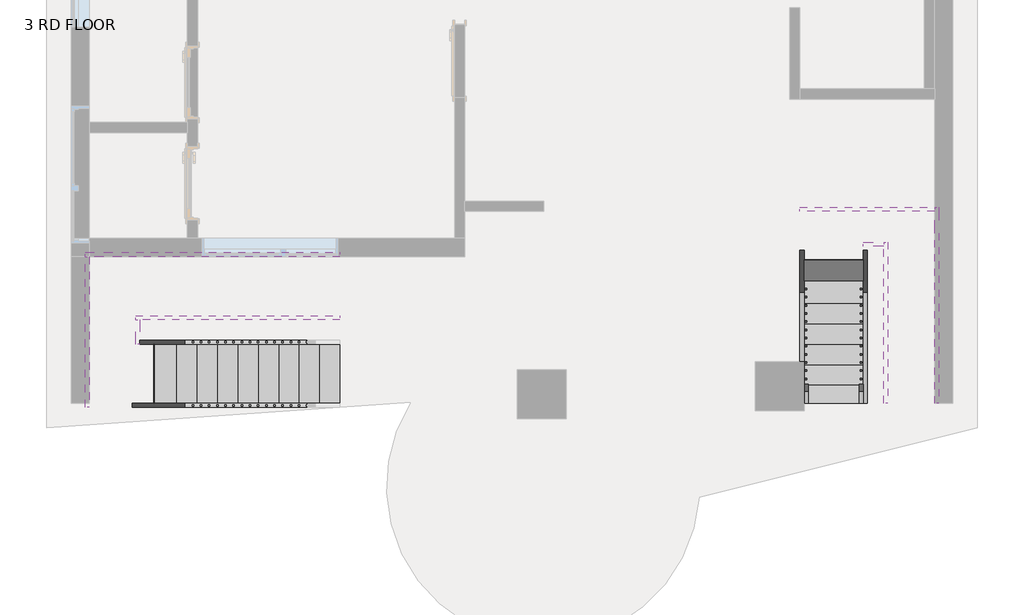
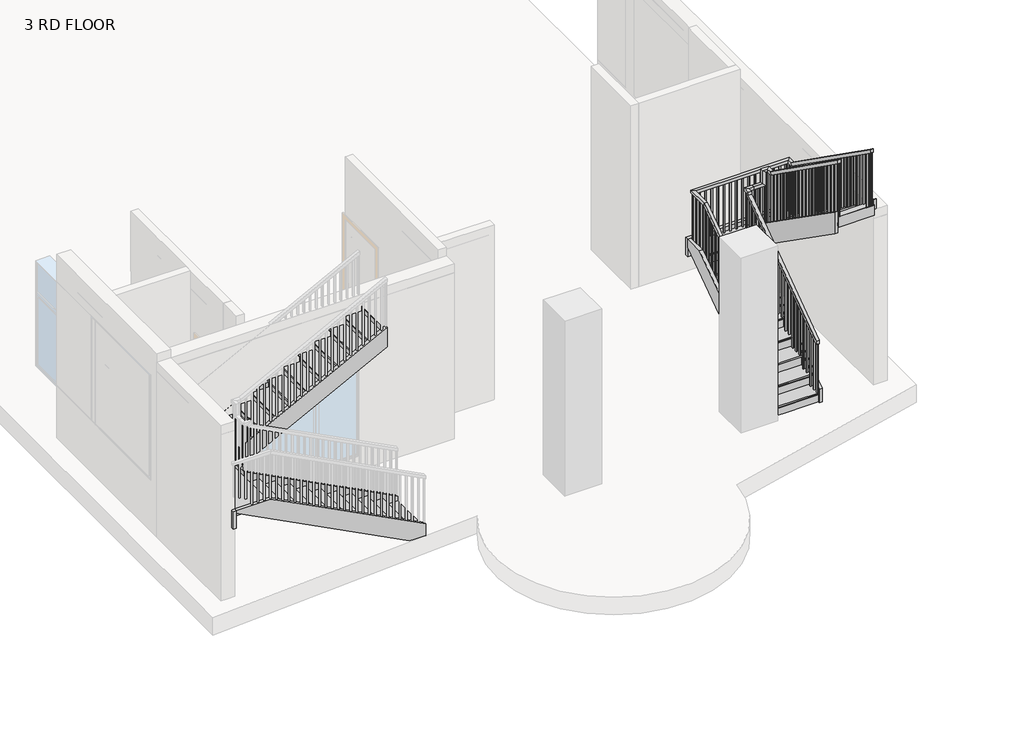
# One storey, part 5 of 5: 12 members, 2 railings, 2 stair flights.
"""IFC4 building model written with IfcOpenShell, lengths in millimetres."""

from ifc_helpers import new_model, si_unit, frame, origin, place, context, project, spatial, polyline, outline, extrude, faceted_brep, transform, mapped, element, save
from components import stair_flight_862ef343, stair_flight_4914edaa

model = new_model("IFC4")

# Units and contexts
model_context = context("Model", 3, world=origin())
ifc_project = project(units=[si_unit("LENGTHUNIT", "METRE", prefix="MILLI")], contexts=[model_context])

# Site, building, storey
site = spatial("IfcSite", under=ifc_project)
building = spatial("IfcBuilding", under=site)
storey = spatial("IfcBuildingStorey", under=building, Name="3 RD FLOOR", Elevation=9601.2)

# Members
placement = place(None, origin())
element("IfcMember", 1, ObjectType="Stringer - 2\" Width", at=placement, inside=storey, context=model_context, shape_type="SweptSolid", body=[
    extrude(outline(polyline([(9601.2, -3117.2664982), (9805.7197081, -3117.2664982), (11125.2, -5663.6319738), (11125.2, -6232.5131972), (11076.6929835, -6232.5131972), (9601.2, -3385.0705974), (9601.2, -3117.2664982)])), frame((0.0, -7701.7822004, 0.0), z_axis=(0.0, 1.0, 0.0), x_axis=(0.0, 0.0, 1.0)), (0.0, 0.0, 1.0), 50.8),
])
element("IfcMember", 2, ObjectType="Stringer - 2\" Width", at=placement, inside=storey, context=model_context, shape_type="SweptSolid", body=[
    extrude(outline(polyline([(-6232.5131972, -7701.7822004), (-6283.3131972, -7701.7822004), (-6283.3131972, -5824.7082131), (-6232.5131972, -5824.7082131), (-6232.5131972, -7701.7822004)])), frame((0.0, 0.0, 10820.4), z_axis=(0.0, 0.0, 1.0), x_axis=(1.0, 0.0, 0.0)), (0.0, 0.0, 1.0), 304.8),
])
element("IfcMember", 3, ObjectType="Stringer - 2\" Width", at=placement, inside=storey, context=model_context, shape_type="SweptSolid", body=[
    extrude(outline(polyline([(10929.1136913, -6283.3131972), (10820.4, -6283.3131972), (10820.4, -5830.6202937), (12226.4106031, -3117.2664982), (12569.7015263, -3117.2664982), (10929.1136913, -6283.3131972)])), frame((0.0, -5824.7082131, 0.0), z_axis=(0.0, 1.0, 0.0), x_axis=(0.0, 0.0, 1.0)), (0.0, 0.0, 1.0), 50.8),
])
element("IfcMember", 4, ObjectType="Stringer - 2\" Width", at=placement, inside=storey, context=model_context, shape_type="SweptSolid", body=[
    extrude(outline(polyline([(9601.2, -3117.2664982), (9805.7197081, -3117.2664982), (11095.5778899, -5606.4664982), (10752.2869668, -5606.4664982), (9601.2, -3385.0705974), (9601.2, -3117.2664982)])), frame((0.0, -6914.3822004, 0.0), z_axis=(0.0, 1.0, 0.0), x_axis=(0.0, 0.0, 1.0)), (0.0, 0.0, 1.0), 50.8),
])
element("IfcMember", 5, ObjectType="Stringer - 2\" Width", at=placement, inside=storey, context=model_context, shape_type="SweptSolid", body=[
    extrude(outline(polyline([(-5606.4664982, -6914.3822004), (-5657.2664982, -6914.3822004), (-5657.2664982, -6609.5822004), (-5606.4664982, -6609.5822004), (-5606.4664982, -6914.3822004)])), frame((0.0, 0.0, 10820.4), z_axis=(0.0, 0.0, 1.0), x_axis=(1.0, 0.0, 0.0)), (0.0, 0.0, 1.0), 304.8),
])
element("IfcMember", 6, ObjectType="Stringer - 2\" Width", at=placement, inside=storey, context=model_context, shape_type="SweptSolid", body=[
    extrude(outline(polyline([(11253.5197081, -5657.2664982), (10910.2287849, -5657.2664982), (12226.4106031, -3117.2664982), (12569.7015263, -3117.2664982), (11253.5197081, -5657.2664982)])), frame((0.0, -6609.5822004, 0.0), z_axis=(0.0, 1.0, 0.0), x_axis=(0.0, 0.0, 1.0)), (0.0, 0.0, 1.0), 50.8),
])
element("IfcMember", 7, ObjectType="Stringer - 2\" Width", at=placement, inside=storey, context=model_context, shape_type="SweptSolid", body=[
    extrude(outline(polyline([(-7650.9822004, 9601.2), (-7650.9822004, 9840.499187), (-5597.981039, 11277.6), (-5263.3822004, 11277.6), (-5263.3822004, 11139.7633718), (-7461.3298744, 9601.2), (-7650.9822004, 9601.2)])), frame((2606.6891134, 0.0, 0.0), z_axis=(1.0, 0.0, 0.0), x_axis=(0.0, 1.0, 0.0)), (0.0, 0.0, 1.0), 50.8),
])
element("IfcMember", 8, ObjectType="Stringer - 2\" Width", at=placement, inside=storey, context=model_context, shape_type="SweptSolid", body=[
    extrude(outline(polyline([(2606.6891134, -5263.3822004), (2606.6891134, -5212.5822004), (4281.7311655, -5212.5822004), (4281.7311655, -5263.3822004), (2606.6891134, -5263.3822004)])), frame((0.0, 0.0, 10972.8), z_axis=(0.0, 0.0, 1.0), x_axis=(1.0, 0.0, 0.0)), (0.0, 0.0, 1.0), 304.8),
])
element("IfcMember", 9, ObjectType="Stringer - 2\" Width", at=placement, inside=storey, context=model_context, shape_type="SweptSolid", body=[
    extrude(outline(polyline([(-5212.5822004, 11120.659187), (-5212.5822004, 10972.8), (-5532.8630978, 10972.8), (-7650.9822004, 12455.4833718), (-7650.9822004, 12827.539187), (-5212.5822004, 11120.659187)])), frame((4281.7311655, 0.0, 0.0), z_axis=(1.0, 0.0, 0.0), x_axis=(0.0, 1.0, 0.0)), (0.0, 0.0, 1.0), 50.8),
])
element("IfcMember", 10, ObjectType="Stringer - 2\" Width", at=placement, inside=storey, context=model_context, shape_type="SweptSolid", body=[
    extrude(outline(polyline([(-7650.9822004, 9601.2), (-7650.9822004, 9840.499187), (-5695.1822004, 11209.559187), (-5695.1822004, 10837.5033718), (-7461.3298744, 9601.2), (-7650.9822004, 9601.2)])), frame((3394.0891134, 0.0, 0.0), z_axis=(1.0, 0.0, 0.0), x_axis=(0.0, 1.0, 0.0)), (0.0, 0.0, 1.0), 50.8),
])
element("IfcMember", 11, ObjectType="Stringer - 2\" Width", at=placement, inside=storey, context=model_context, shape_type="SweptSolid", body=[
    extrude(outline(polyline([(3394.0891134, -5695.1822004), (3394.0891134, -5644.3822004), (3648.0891134, -5644.3822004), (3648.0891134, -5695.1822004), (3394.0891134, -5695.1822004)])), frame((0.0, 0.0, 10972.8), z_axis=(0.0, 0.0, 1.0), x_axis=(1.0, 0.0, 0.0)), (0.0, 0.0, 1.0), 304.8),
])
element("IfcMember", 12, ObjectType="Stringer - 2\" Width", at=placement, inside=storey, context=model_context, shape_type="SweptSolid", body=[
    extrude(outline(polyline([(-5644.3822004, 11422.919187), (-5644.3822004, 11050.8633718), (-7650.9822004, 12455.4833718), (-7650.9822004, 12827.539187), (-5644.3822004, 11422.919187)])), frame((3648.0891134, 0.0, 0.0), z_axis=(1.0, 0.0, 0.0), x_axis=(0.0, 1.0, 0.0)), (0.0, 0.0, 1.0), 50.8),
])

# Railings
element("IfcRailing", 13, ObjectType="Handrail - Rectangular", at=placement, inside=storey, context=model_context, shape_type="SolidModel", body=[
    faceted_brep([(3343.2891134, -7650.9822004, 10693.4), (3343.2891134, -7650.9822004, 10631.1314749), (3394.0891134, -7650.9822004, 10631.1314749), (3394.0891134, -7650.9822004, 10693.4), (3343.2891134, -5720.5822004, 12061.7848101), (3343.2891134, -5669.7822004, 12035.5264116), (3394.0891134, -5669.7822004, 12035.5264116), (3394.0891134, -5720.5822004, 12061.7848101), (3343.2891134, -5720.5822004, 12115.8), (3343.2891134, -5669.7822004, 12065.0), (3394.0891134, -5669.7822004, 12065.0), (3394.0891134, -5720.5822004, 12115.8), (3343.2891134, -5593.5822004, 12115.8), (3343.2891134, -5593.5822004, 12065.0), (3394.0891134, -5644.3822004, 12065.0), (3394.0891134, -5644.3822004, 12115.8), (3470.2891134, -5593.5822004, 12115.8), (3470.2891134, -5593.5822004, 12065.0), (3470.2891134, -5644.3822004, 12065.0), (3470.2891134, -5644.3822004, 12115.8), (3622.6891134, -5593.5822004, 12115.8), (3673.4891134, -5593.5822004, 12065.0), (3673.4891134, -5644.3822004, 12065.0), (3622.6891134, -5644.3822004, 12115.8), (3622.6891134, -5593.5822004, 12347.6151899), (3673.4891134, -5593.5822004, 12296.8151899), (3673.4891134, -5644.3822004, 12296.8151899), (3622.6891134, -5644.3822004, 12347.6151899), (3749.6891134, -5593.5822004, 12347.6151899), (3749.6891134, -5593.5822004, 12296.8151899), (3698.8891134, -5644.3822004, 12296.8151899), (3698.8891134, -5644.3822004, 12347.6151899), (3749.6891134, -5720.5822004, 12347.6151899), (3749.6891134, -5736.7610126, 12296.8151899), (3698.8891134, -5736.7610126, 12296.8151899), (3698.8891134, -5720.5822004, 12347.6151899), (3749.6891134, -7650.9822004, 13716.0), (3698.8891134, -7650.9822004, 13716.0), (3698.8891134, -7650.9822004, 13653.7314749), (3749.6891134, -7650.9822004, 13653.7314749)], [[[0, 1, 2, 3]], [[1, 0, 4, 5]], [[2, 1, 5, 6]], [[3, 2, 6, 7]], [[0, 3, 7, 4]], [[5, 4, 8, 9]], [[6, 5, 9, 10]], [[7, 6, 10, 11]], [[4, 7, 11, 8]], [[9, 8, 12, 13]], [[10, 9, 13, 14]], [[11, 10, 14, 15]], [[8, 11, 15, 12]], [[13, 12, 16, 17]], [[14, 13, 17, 18]], [[15, 14, 18, 19]], [[12, 15, 19, 16]], [[17, 16, 20, 21]], [[18, 17, 21, 22]], [[19, 18, 22, 23]], [[16, 19, 23, 20]], [[21, 20, 24, 25]], [[22, 21, 25, 26]], [[23, 22, 26, 27]], [[20, 23, 27, 24]], [[25, 24, 28, 29]], [[26, 25, 29, 30]], [[27, 26, 30, 31]], [[24, 27, 31, 28]], [[29, 28, 32, 33]], [[30, 29, 33, 34]], [[31, 30, 34, 35]], [[28, 31, 35, 32]], [[36, 37, 38, 39]], [[33, 32, 36, 39]], [[34, 33, 39, 38]], [[35, 34, 38, 37]], [[32, 35, 37, 36]]]),
    extrude(outline(polyline([(-7558.9072004, 13588.4631205), (-7539.8572004, 13574.959323), (-7539.8572004, 12623.8), (-7558.9072004, 12623.8), (-7558.9072004, 13588.4631205)])), frame((3714.7641134, 0.0, 0.0), z_axis=(1.0, 0.0, 0.0), x_axis=(0.0, 1.0, 0.0)), (0.0, 0.0, 1.0), 19.05),
    extrude(outline(polyline([(-7457.3072004, 13516.4428673), (-7438.2572004, 13502.9390699), (-7438.2572004, 12623.8), (-7457.3072004, 12623.8), (-7457.3072004, 13516.4428673)])), frame((3714.7641134, 0.0, 0.0), z_axis=(1.0, 0.0, 0.0), x_axis=(0.0, 1.0, 0.0)), (0.0, 0.0, 1.0), 19.05),
    extrude(outline(polyline([(-7355.7072004, 13444.4226142), (-7336.6572004, 13430.9188167), (-7336.6572004, 12446.0), (-7355.7072004, 12446.0), (-7355.7072004, 13444.4226142)])), frame((3714.7641134, 0.0, 0.0), z_axis=(1.0, 0.0, 0.0), x_axis=(0.0, 1.0, 0.0)), (0.0, 0.0, 1.0), 19.05),
    extrude(outline(polyline([(-7254.1072004, 13372.402361), (-7235.0572004, 13358.8985635), (-7235.0572004, 12446.0), (-7254.1072004, 12446.0), (-7254.1072004, 13372.402361)])), frame((3714.7641134, 0.0, 0.0), z_axis=(1.0, 0.0, 0.0), x_axis=(0.0, 1.0, 0.0)), (0.0, 0.0, 1.0), 19.05),
    extrude(outline(polyline([(-7152.5072004, 13300.3821078), (-7133.4572004, 13286.8783104), (-7133.4572004, 12268.2), (-7152.5072004, 12268.2), (-7152.5072004, 13300.3821078)])), frame((3714.7641134, 0.0, 0.0), z_axis=(1.0, 0.0, 0.0), x_axis=(0.0, 1.0, 0.0)), (0.0, 0.0, 1.0), 19.05),
    extrude(outline(polyline([(-7050.9072004, 13228.3618547), (-7031.8572004, 13214.8580572), (-7031.8572004, 12268.2), (-7050.9072004, 12268.2), (-7050.9072004, 13228.3618547)])), frame((3714.7641134, 0.0, 0.0), z_axis=(1.0, 0.0, 0.0), x_axis=(0.0, 1.0, 0.0)), (0.0, 0.0, 1.0), 19.05),
    extrude(outline(polyline([(-6949.3072004, 13156.3416015), (-6930.2572004, 13142.837804), (-6930.2572004, 12268.2), (-6949.3072004, 12268.2), (-6949.3072004, 13156.3416015)])), frame((3714.7641134, 0.0, 0.0), z_axis=(1.0, 0.0, 0.0), x_axis=(0.0, 1.0, 0.0)), (0.0, 0.0, 1.0), 19.05),
    extrude(outline(polyline([(-6847.7072004, 13084.3213483), (-6828.6572004, 13070.8175509), (-6828.6572004, 12090.4), (-6847.7072004, 12090.4), (-6847.7072004, 13084.3213483)])), frame((3714.7641134, 0.0, 0.0), z_axis=(1.0, 0.0, 0.0), x_axis=(0.0, 1.0, 0.0)), (0.0, 0.0, 1.0), 19.05),
    extrude(outline(polyline([(-6746.1072004, 13012.3010952), (-6727.0572004, 12998.7972977), (-6727.0572004, 12090.4), (-6746.1072004, 12090.4), (-6746.1072004, 13012.3010952)])), frame((3714.7641134, 0.0, 0.0), z_axis=(1.0, 0.0, 0.0), x_axis=(0.0, 1.0, 0.0)), (0.0, 0.0, 1.0), 19.05),
    extrude(outline(polyline([(-6644.5072004, 12940.280842), (-6625.4572004, 12926.7770445), (-6625.4572004, 11912.6), (-6644.5072004, 11912.6), (-6644.5072004, 12940.280842)])), frame((3714.7641134, 0.0, 0.0), z_axis=(1.0, 0.0, 0.0), x_axis=(0.0, 1.0, 0.0)), (0.0, 0.0, 1.0), 19.05),
    extrude(outline(polyline([(-6542.9072004, 12868.2605888), (-6523.8572004, 12854.7567914), (-6523.8572004, 11912.6), (-6542.9072004, 11912.6), (-6542.9072004, 12868.2605888)])), frame((3714.7641134, 0.0, 0.0), z_axis=(1.0, 0.0, 0.0), x_axis=(0.0, 1.0, 0.0)), (0.0, 0.0, 1.0), 19.05),
    extrude(outline(polyline([(-6441.3072004, 12796.2403357), (-6422.2572004, 12782.7365382), (-6422.2572004, 11912.6), (-6441.3072004, 11912.6), (-6441.3072004, 12796.2403357)])), frame((3714.7641134, 0.0, 0.0), z_axis=(1.0, 0.0, 0.0), x_axis=(0.0, 1.0, 0.0)), (0.0, 0.0, 1.0), 19.05),
    extrude(outline(polyline([(-6339.7072004, 12724.2200825), (-6320.6572004, 12710.716285), (-6320.6572004, 11734.8), (-6339.7072004, 11734.8), (-6339.7072004, 12724.2200825)])), frame((3714.7641134, 0.0, 0.0), z_axis=(1.0, 0.0, 0.0), x_axis=(0.0, 1.0, 0.0)), (0.0, 0.0, 1.0), 19.05),
    extrude(outline(polyline([(-6238.1072004, 12652.1998293), (-6219.0572004, 12638.6960319), (-6219.0572004, 11734.8), (-6238.1072004, 11734.8), (-6238.1072004, 12652.1998293)])), frame((3714.7641134, 0.0, 0.0), z_axis=(1.0, 0.0, 0.0), x_axis=(0.0, 1.0, 0.0)), (0.0, 0.0, 1.0), 19.05),
    extrude(outline(polyline([(-6136.5072004, 12580.1795762), (-6117.4572004, 12566.6757787), (-6117.4572004, 11557.0), (-6136.5072004, 11557.0), (-6136.5072004, 12580.1795762)])), frame((3714.7641134, 0.0, 0.0), z_axis=(1.0, 0.0, 0.0), x_axis=(0.0, 1.0, 0.0)), (0.0, 0.0, 1.0), 19.05),
    extrude(outline(polyline([(-6034.9072004, 12508.159323), (-6015.8572004, 12494.6555255), (-6015.8572004, 11557.0), (-6034.9072004, 11557.0), (-6034.9072004, 12508.159323)])), frame((3714.7641134, 0.0, 0.0), z_axis=(1.0, 0.0, 0.0), x_axis=(0.0, 1.0, 0.0)), (0.0, 0.0, 1.0), 19.05),
    extrude(outline(polyline([(-5933.3072004, 12436.1390699), (-5914.2572004, 12422.6352724), (-5914.2572004, 11557.0), (-5933.3072004, 11557.0), (-5933.3072004, 12436.1390699)])), frame((3714.7641134, 0.0, 0.0), z_axis=(1.0, 0.0, 0.0), x_axis=(0.0, 1.0, 0.0)), (0.0, 0.0, 1.0), 19.05),
    extrude(outline(polyline([(-5831.7072004, 12364.1188167), (-5812.6572004, 12350.6150192), (-5812.6572004, 11379.2), (-5831.7072004, 11379.2), (-5831.7072004, 12364.1188167)])), frame((3714.7641134, 0.0, 0.0), z_axis=(1.0, 0.0, 0.0), x_axis=(0.0, 1.0, 0.0)), (0.0, 0.0, 1.0), 19.05),
    extrude(outline(polyline([(-5730.1072004, 12292.0985635), (-5711.0572004, 12278.5947661), (-5711.0572004, 11379.2), (-5730.1072004, 11379.2), (-5730.1072004, 12292.0985635)])), frame((3714.7641134, 0.0, 0.0), z_axis=(1.0, 0.0, 0.0), x_axis=(0.0, 1.0, 0.0)), (0.0, 0.0, 1.0), 19.05),
    extrude(outline(polyline([(3663.9641134, -5628.5072004), (3663.9641134, -5609.4572004), (3683.0141134, -5609.4572004), (3683.0141134, -5628.5072004), (3663.9641134, -5628.5072004)])), frame((0.0, 0.0, 11201.4), z_axis=(0.0, 0.0, 1.0), x_axis=(1.0, 0.0, 0.0)), (0.0, 0.0, 1.0), 1095.4151899),
    extrude(outline(polyline([(3562.3641134, -5628.5072004), (3562.3641134, -5609.4572004), (3581.4141134, -5609.4572004), (3581.4141134, -5628.5072004), (3562.3641134, -5628.5072004)])), frame((0.0, 0.0, 11201.4), z_axis=(0.0, 0.0, 1.0), x_axis=(1.0, 0.0, 0.0)), (0.0, 0.0, 1.0), 863.6),
    extrude(outline(polyline([(3460.7641134, -5628.5072004), (3460.7641134, -5609.4572004), (3479.8141134, -5609.4572004), (3479.8141134, -5628.5072004), (3460.7641134, -5628.5072004)])), frame((0.0, 0.0, 11201.4), z_axis=(0.0, 0.0, 1.0), x_axis=(1.0, 0.0, 0.0)), (0.0, 0.0, 1.0), 863.6),
    extrude(outline(polyline([(-5730.1072004, 11992.7643863), (-5711.0572004, 12006.2681838), (-5711.0572004, 11023.6), (-5730.1072004, 11023.6), (-5730.1072004, 11992.7643863)])), frame((3359.1641134, 0.0, 0.0), z_axis=(1.0, 0.0, 0.0), x_axis=(0.0, 1.0, 0.0)), (0.0, 0.0, 1.0), 19.05),
    extrude(outline(polyline([(-5831.7072004, 11920.7441331), (-5812.6572004, 11934.2479306), (-5812.6572004, 11023.6), (-5831.7072004, 11023.6), (-5831.7072004, 11920.7441331)])), frame((3359.1641134, 0.0, 0.0), z_axis=(1.0, 0.0, 0.0), x_axis=(0.0, 1.0, 0.0)), (0.0, 0.0, 1.0), 19.05),
    extrude(outline(polyline([(-5933.3072004, 11848.72388), (-5914.2572004, 11862.2276774), (-5914.2572004, 10845.8), (-5933.3072004, 10845.8), (-5933.3072004, 11848.72388)])), frame((3359.1641134, 0.0, 0.0), z_axis=(1.0, 0.0, 0.0), x_axis=(0.0, 1.0, 0.0)), (0.0, 0.0, 1.0), 19.05),
    extrude(outline(polyline([(-6034.9072004, 11776.7036268), (-6015.8572004, 11790.2074243), (-6015.8572004, 10845.8), (-6034.9072004, 10845.8), (-6034.9072004, 11776.7036268)])), frame((3359.1641134, 0.0, 0.0), z_axis=(1.0, 0.0, 0.0), x_axis=(0.0, 1.0, 0.0)), (0.0, 0.0, 1.0), 19.05),
    extrude(outline(polyline([(-6136.5072004, 11704.6833736), (-6117.4572004, 11718.1871711), (-6117.4572004, 10845.8), (-6136.5072004, 10845.8), (-6136.5072004, 11704.6833736)])), frame((3359.1641134, 0.0, 0.0), z_axis=(1.0, 0.0, 0.0), x_axis=(0.0, 1.0, 0.0)), (0.0, 0.0, 1.0), 19.05),
    extrude(outline(polyline([(-6238.1072004, 11632.6631205), (-6219.0572004, 11646.166918), (-6219.0572004, 10668.0), (-6238.1072004, 10668.0), (-6238.1072004, 11632.6631205)])), frame((3359.1641134, 0.0, 0.0), z_axis=(1.0, 0.0, 0.0), x_axis=(0.0, 1.0, 0.0)), (0.0, 0.0, 1.0), 19.05),
    extrude(outline(polyline([(-6339.7072004, 11560.6428673), (-6320.6572004, 11574.1466648), (-6320.6572004, 10668.0), (-6339.7072004, 10668.0), (-6339.7072004, 11560.6428673)])), frame((3359.1641134, 0.0, 0.0), z_axis=(1.0, 0.0, 0.0), x_axis=(0.0, 1.0, 0.0)), (0.0, 0.0, 1.0), 19.05),
    extrude(outline(polyline([(-6441.3072004, 11488.6226142), (-6422.2572004, 11502.1264116), (-6422.2572004, 10490.2), (-6441.3072004, 10490.2), (-6441.3072004, 11488.6226142)])), frame((3359.1641134, 0.0, 0.0), z_axis=(1.0, 0.0, 0.0), x_axis=(0.0, 1.0, 0.0)), (0.0, 0.0, 1.0), 19.05),
    extrude(outline(polyline([(-6542.9072004, 11416.602361), (-6523.8572004, 11430.1061585), (-6523.8572004, 10490.2), (-6542.9072004, 10490.2), (-6542.9072004, 11416.602361)])), frame((3359.1641134, 0.0, 0.0), z_axis=(1.0, 0.0, 0.0), x_axis=(0.0, 1.0, 0.0)), (0.0, 0.0, 1.0), 19.05),
    extrude(outline(polyline([(-6644.5072004, 11344.5821078), (-6625.4572004, 11358.0859053), (-6625.4572004, 10490.2), (-6644.5072004, 10490.2), (-6644.5072004, 11344.5821078)])), frame((3359.1641134, 0.0, 0.0), z_axis=(1.0, 0.0, 0.0), x_axis=(0.0, 1.0, 0.0)), (0.0, 0.0, 1.0), 19.05),
    extrude(outline(polyline([(-6746.1072004, 11272.5618547), (-6727.0572004, 11286.0656521), (-6727.0572004, 10312.4), (-6746.1072004, 10312.4), (-6746.1072004, 11272.5618547)])), frame((3359.1641134, 0.0, 0.0), z_axis=(1.0, 0.0, 0.0), x_axis=(0.0, 1.0, 0.0)), (0.0, 0.0, 1.0), 19.05),
    extrude(outline(polyline([(-6847.7072004, 11200.5416015), (-6828.6572004, 11214.045399), (-6828.6572004, 10312.4), (-6847.7072004, 10312.4), (-6847.7072004, 11200.5416015)])), frame((3359.1641134, 0.0, 0.0), z_axis=(1.0, 0.0, 0.0), x_axis=(0.0, 1.0, 0.0)), (0.0, 0.0, 1.0), 19.05),
    extrude(outline(polyline([(-6949.3072004, 11128.5213483), (-6930.2572004, 11142.0251458), (-6930.2572004, 10134.6), (-6949.3072004, 10134.6), (-6949.3072004, 11128.5213483)])), frame((3359.1641134, 0.0, 0.0), z_axis=(1.0, 0.0, 0.0), x_axis=(0.0, 1.0, 0.0)), (0.0, 0.0, 1.0), 19.05),
    extrude(outline(polyline([(-7050.9072004, 11056.5010952), (-7031.8572004, 11070.0048926), (-7031.8572004, 10134.6), (-7050.9072004, 10134.6), (-7050.9072004, 11056.5010952)])), frame((3359.1641134, 0.0, 0.0), z_axis=(1.0, 0.0, 0.0), x_axis=(0.0, 1.0, 0.0)), (0.0, 0.0, 1.0), 19.05),
    extrude(outline(polyline([(-7152.5072004, 10984.480842), (-7133.4572004, 10997.9846395), (-7133.4572004, 10134.6), (-7152.5072004, 10134.6), (-7152.5072004, 10984.480842)])), frame((3359.1641134, 0.0, 0.0), z_axis=(1.0, 0.0, 0.0), x_axis=(0.0, 1.0, 0.0)), (0.0, 0.0, 1.0), 19.05),
    extrude(outline(polyline([(-7254.1072004, 10912.4605888), (-7235.0572004, 10925.9643863), (-7235.0572004, 9956.8), (-7254.1072004, 9956.8), (-7254.1072004, 10912.4605888)])), frame((3359.1641134, 0.0, 0.0), z_axis=(1.0, 0.0, 0.0), x_axis=(0.0, 1.0, 0.0)), (0.0, 0.0, 1.0), 19.05),
    extrude(outline(polyline([(-7355.7072004, 10840.4403357), (-7336.6572004, 10853.9441331), (-7336.6572004, 9956.8), (-7355.7072004, 9956.8), (-7355.7072004, 10840.4403357)])), frame((3359.1641134, 0.0, 0.0), z_axis=(1.0, 0.0, 0.0), x_axis=(0.0, 1.0, 0.0)), (0.0, 0.0, 1.0), 19.05),
    extrude(outline(polyline([(-7457.3072004, 10768.4200825), (-7438.2572004, 10781.92388), (-7438.2572004, 9779.0), (-7457.3072004, 9779.0), (-7457.3072004, 10768.4200825)])), frame((3359.1641134, 0.0, 0.0), z_axis=(1.0, 0.0, 0.0), x_axis=(0.0, 1.0, 0.0)), (0.0, 0.0, 1.0), 19.05),
    extrude(outline(polyline([(-7558.9072004, 10696.3998293), (-7539.8572004, 10709.9036268), (-7539.8572004, 9779.0), (-7558.9072004, 9779.0), (-7558.9072004, 10696.3998293)])), frame((3359.1641134, 0.0, 0.0), z_axis=(1.0, 0.0, 0.0), x_axis=(0.0, 1.0, 0.0)), (0.0, 0.0, 1.0), 19.05),
    extrude(outline(polyline([(3714.7641134, -5628.5072004), (3714.7641134, -5609.4572004), (3733.8141134, -5609.4572004), (3733.8141134, -5628.5072004), (3714.7641134, -5628.5072004)])), frame((0.0, 0.0, 11201.4), z_axis=(0.0, 0.0, 1.0), x_axis=(1.0, 0.0, 0.0)), (0.0, 0.0, 1.0), 1095.4151899),
    extrude(outline(polyline([(3378.2141134, -5628.5072004), (3359.1641134, -5628.5072004), (3359.1641134, -5609.4572004), (3378.2141134, -5609.4572004), (3378.2141134, -5628.5072004)])), frame((0.0, 0.0, 11201.4), z_axis=(0.0, 0.0, 1.0), x_axis=(1.0, 0.0, 0.0)), (0.0, 0.0, 1.0), 863.6),
    extrude(outline(polyline([(-7650.9822004, 13653.7314749), (-7631.9322004, 13640.2276774), (-7631.9322004, 12623.8), (-7650.9822004, 12623.8), (-7650.9822004, 13653.7314749)])), frame((3714.7641134, 0.0, 0.0), z_axis=(1.0, 0.0, 0.0), x_axis=(0.0, 1.0, 0.0)), (0.0, 0.0, 1.0), 19.05),
    extrude(outline(polyline([(-7650.9822004, 10631.1314749), (-7631.9322004, 10644.6352724), (-7631.9322004, 9779.0), (-7650.9822004, 9779.0), (-7650.9822004, 10631.1314749)])), frame((3359.1641134, 0.0, 0.0), z_axis=(1.0, 0.0, 0.0), x_axis=(0.0, 1.0, 0.0)), (0.0, 0.0, 1.0), 19.05),
])
element("IfcRailing", 14, ObjectType="Handrail - Rectangular", at=placement, inside=storey, context=model_context, shape_type="SolidModel", body=[
    faceted_brep([(2657.4891134, -7650.9822004, 10693.4), (2657.4891134, -7650.9822004, 10631.1314749), (2708.2891134, -7650.9822004, 10631.1314749), (2708.2891134, -7650.9822004, 10693.4), (2657.4891134, -5644.3822004, 12115.8), (2657.4891134, -5628.2033882, 12065.0), (2708.2891134, -5628.2033882, 12065.0), (2708.2891134, -5644.3822004, 12115.8), (2657.4891134, -5263.3822004, 12115.8), (2657.4891134, -5263.3822004, 12065.0), (2708.2891134, -5314.1822004, 12065.0), (2708.2891134, -5314.1822004, 12115.8), (4281.7311655, -5263.3822004, 12115.8), (4281.7311655, -5263.3822004, 12065.0), (4230.9311655, -5314.1822004, 12065.0), (4230.9311655, -5314.1822004, 12115.8), (4281.7311655, -5393.5572004, 12115.8), (4281.7311655, -5409.7360126, 12065.0), (4230.9311655, -5409.7360126, 12065.0), (4230.9311655, -5393.5572004, 12115.8), (4281.7311655, -7650.9822004, 13716.0), (4230.9311655, -7650.9822004, 13716.0), (4230.9311655, -7650.9822004, 13653.7314749), (4281.7311655, -7650.9822004, 13653.7314749)], [[[0, 1, 2, 3]], [[1, 0, 4, 5]], [[2, 1, 5, 6]], [[3, 2, 6, 7]], [[0, 3, 7, 4]], [[5, 4, 8, 9]], [[6, 5, 9, 10]], [[7, 6, 10, 11]], [[4, 7, 11, 8]], [[9, 8, 12, 13]], [[10, 9, 13, 14]], [[11, 10, 14, 15]], [[8, 11, 15, 12]], [[13, 12, 16, 17]], [[14, 13, 17, 18]], [[15, 14, 18, 19]], [[12, 15, 19, 16]], [[20, 21, 22, 23]], [[17, 16, 20, 23]], [[18, 17, 23, 22]], [[19, 18, 22, 21]], [[16, 19, 21, 20]]]),
    extrude(outline(polyline([(-7616.0572004, 13628.9745129), (-7616.0572004, 12623.8), (-7635.1072004, 12623.8), (-7635.1072004, 13642.4783104), (-7616.0572004, 13628.9745129)])), frame((4246.8061655, 0.0, 0.0), z_axis=(1.0, 0.0, 0.0), x_axis=(0.0, 1.0, 0.0)), (0.0, 0.0, 1.0), 19.05),
    extrude(outline(polyline([(-7514.4572004, 13556.9542597), (-7514.4572004, 12623.8), (-7533.5072004, 12623.8), (-7533.5072004, 13570.4580572), (-7514.4572004, 13556.9542597)])), frame((4246.8061655, 0.0, 0.0), z_axis=(1.0, 0.0, 0.0), x_axis=(0.0, 1.0, 0.0)), (0.0, 0.0, 1.0), 19.05),
    extrude(outline(polyline([(-7412.8572004, 13484.9340066), (-7412.8572004, 12623.8), (-7431.9072004, 12623.8), (-7431.9072004, 13498.437804), (-7412.8572004, 13484.9340066)])), frame((4246.8061655, 0.0, 0.0), z_axis=(1.0, 0.0, 0.0), x_axis=(0.0, 1.0, 0.0)), (0.0, 0.0, 1.0), 19.05),
    extrude(outline(polyline([(-7311.2572004, 13412.9137534), (-7311.2572004, 12446.0), (-7330.3072004, 12446.0), (-7330.3072004, 13426.4175509), (-7311.2572004, 13412.9137534)])), frame((4246.8061655, 0.0, 0.0), z_axis=(1.0, 0.0, 0.0), x_axis=(0.0, 1.0, 0.0)), (0.0, 0.0, 1.0), 19.05),
    extrude(outline(polyline([(-7209.6572004, 13340.8935002), (-7209.6572004, 12446.0), (-7228.7072004, 12446.0), (-7228.7072004, 13354.3972977), (-7209.6572004, 13340.8935002)])), frame((4246.8061655, 0.0, 0.0), z_axis=(1.0, 0.0, 0.0), x_axis=(0.0, 1.0, 0.0)), (0.0, 0.0, 1.0), 19.05),
    extrude(outline(polyline([(-7108.0572004, 13268.8732471), (-7108.0572004, 12268.2), (-7127.1072004, 12268.2), (-7127.1072004, 13282.3770445), (-7108.0572004, 13268.8732471)])), frame((4246.8061655, 0.0, 0.0), z_axis=(1.0, 0.0, 0.0), x_axis=(0.0, 1.0, 0.0)), (0.0, 0.0, 1.0), 19.05),
    extrude(outline(polyline([(-7006.4572004, 13196.8529939), (-7006.4572004, 12268.2), (-7025.5072004, 12268.2), (-7025.5072004, 13210.3567914), (-7006.4572004, 13196.8529939)])), frame((4246.8061655, 0.0, 0.0), z_axis=(1.0, 0.0, 0.0), x_axis=(0.0, 1.0, 0.0)), (0.0, 0.0, 1.0), 19.05),
    extrude(outline(polyline([(-6904.8572004, 13124.8327407), (-6904.8572004, 12268.2), (-6923.9072004, 12268.2), (-6923.9072004, 13138.3365382), (-6904.8572004, 13124.8327407)])), frame((4246.8061655, 0.0, 0.0), z_axis=(1.0, 0.0, 0.0), x_axis=(0.0, 1.0, 0.0)), (0.0, 0.0, 1.0), 19.05),
    extrude(outline(polyline([(-6803.2572004, 13052.8124876), (-6803.2572004, 12090.4), (-6822.3072004, 12090.4), (-6822.3072004, 13066.316285), (-6803.2572004, 13052.8124876)])), frame((4246.8061655, 0.0, 0.0), z_axis=(1.0, 0.0, 0.0), x_axis=(0.0, 1.0, 0.0)), (0.0, 0.0, 1.0), 19.05),
    extrude(outline(polyline([(-6701.6572004, 12980.7922344), (-6701.6572004, 12090.4), (-6720.7072004, 12090.4), (-6720.7072004, 12994.2960319), (-6701.6572004, 12980.7922344)])), frame((4246.8061655, 0.0, 0.0), z_axis=(1.0, 0.0, 0.0), x_axis=(0.0, 1.0, 0.0)), (0.0, 0.0, 1.0), 19.05),
    extrude(outline(polyline([(-6600.0572004, 12908.7719812), (-6600.0572004, 11912.6), (-6619.1072004, 11912.6), (-6619.1072004, 12922.2757787), (-6600.0572004, 12908.7719812)])), frame((4246.8061655, 0.0, 0.0), z_axis=(1.0, 0.0, 0.0), x_axis=(0.0, 1.0, 0.0)), (0.0, 0.0, 1.0), 19.05),
    extrude(outline(polyline([(-6498.4572004, 12836.7517281), (-6498.4572004, 11912.6), (-6517.5072004, 11912.6), (-6517.5072004, 12850.2555255), (-6498.4572004, 12836.7517281)])), frame((4246.8061655, 0.0, 0.0), z_axis=(1.0, 0.0, 0.0), x_axis=(0.0, 1.0, 0.0)), (0.0, 0.0, 1.0), 19.05),
    extrude(outline(polyline([(-6396.8572004, 12764.7314749), (-6396.8572004, 11912.6), (-6415.9072004, 11912.6), (-6415.9072004, 12778.2352724), (-6396.8572004, 12764.7314749)])), frame((4246.8061655, 0.0, 0.0), z_axis=(1.0, 0.0, 0.0), x_axis=(0.0, 1.0, 0.0)), (0.0, 0.0, 1.0), 19.05),
    extrude(outline(polyline([(-6295.2572004, 12692.7112217), (-6295.2572004, 11734.8), (-6314.3072004, 11734.8), (-6314.3072004, 12706.2150192), (-6295.2572004, 12692.7112217)])), frame((4246.8061655, 0.0, 0.0), z_axis=(1.0, 0.0, 0.0), x_axis=(0.0, 1.0, 0.0)), (0.0, 0.0, 1.0), 19.05),
    extrude(outline(polyline([(-6193.6572004, 12620.6909686), (-6193.6572004, 11734.8), (-6212.7072004, 11734.8), (-6212.7072004, 12634.1947661), (-6193.6572004, 12620.6909686)])), frame((4246.8061655, 0.0, 0.0), z_axis=(1.0, 0.0, 0.0), x_axis=(0.0, 1.0, 0.0)), (0.0, 0.0, 1.0), 19.05),
    extrude(outline(polyline([(-6092.0572004, 12548.6707154), (-6092.0572004, 11557.0), (-6111.1072004, 11557.0), (-6111.1072004, 12562.1745129), (-6092.0572004, 12548.6707154)])), frame((4246.8061655, 0.0, 0.0), z_axis=(1.0, 0.0, 0.0), x_axis=(0.0, 1.0, 0.0)), (0.0, 0.0, 1.0), 19.05),
    extrude(outline(polyline([(-5990.4572004, 12476.6504623), (-5990.4572004, 11557.0), (-6009.5072004, 11557.0), (-6009.5072004, 12490.1542597), (-5990.4572004, 12476.6504623)])), frame((4246.8061655, 0.0, 0.0), z_axis=(1.0, 0.0, 0.0), x_axis=(0.0, 1.0, 0.0)), (0.0, 0.0, 1.0), 19.05),
    extrude(outline(polyline([(-5888.8572004, 12404.6302091), (-5888.8572004, 11557.0), (-5907.9072004, 11557.0), (-5907.9072004, 12418.1340066), (-5888.8572004, 12404.6302091)])), frame((4246.8061655, 0.0, 0.0), z_axis=(1.0, 0.0, 0.0), x_axis=(0.0, 1.0, 0.0)), (0.0, 0.0, 1.0), 19.05),
    extrude(outline(polyline([(-5787.2572004, 12332.6099559), (-5787.2572004, 11379.2), (-5806.3072004, 11379.2), (-5806.3072004, 12346.1137534), (-5787.2572004, 12332.6099559)])), frame((4246.8061655, 0.0, 0.0), z_axis=(1.0, 0.0, 0.0), x_axis=(0.0, 1.0, 0.0)), (0.0, 0.0, 1.0), 19.05),
    extrude(outline(polyline([(-5685.6572004, 12260.5897028), (-5685.6572004, 11379.2), (-5704.7072004, 11379.2), (-5704.7072004, 12274.0935002), (-5685.6572004, 12260.5897028)])), frame((4246.8061655, 0.0, 0.0), z_axis=(1.0, 0.0, 0.0), x_axis=(0.0, 1.0, 0.0)), (0.0, 0.0, 1.0), 19.05),
    extrude(outline(polyline([(-5584.0572004, 12188.5694496), (-5584.0572004, 11201.4), (-5603.1072004, 11201.4), (-5603.1072004, 12202.0732471), (-5584.0572004, 12188.5694496)])), frame((4246.8061655, 0.0, 0.0), z_axis=(1.0, 0.0, 0.0), x_axis=(0.0, 1.0, 0.0)), (0.0, 0.0, 1.0), 19.05),
    extrude(outline(polyline([(-5482.4572004, 12116.5491964), (-5482.4572004, 11201.4), (-5501.5072004, 11201.4), (-5501.5072004, 12130.0529939), (-5482.4572004, 12116.5491964)])), frame((4246.8061655, 0.0, 0.0), z_axis=(1.0, 0.0, 0.0), x_axis=(0.0, 1.0, 0.0)), (0.0, 0.0, 1.0), 19.05),
    extrude(outline(polyline([(4265.8561655, -5380.8572004), (4265.8561655, -5399.9072004), (4246.8061655, -5399.9072004), (4246.8061655, -5380.8572004), (4265.8561655, -5380.8572004)])), frame((0.0, 0.0, 11201.4), z_axis=(0.0, 0.0, 1.0), x_axis=(1.0, 0.0, 0.0)), (0.0, 0.0, 1.0), 863.6),
    extrude(outline(polyline([(4197.3641134, -5279.2572004), (4216.4141134, -5279.2572004), (4216.4141134, -5298.3072004), (4197.3641134, -5298.3072004), (4197.3641134, -5279.2572004)])), frame((0.0, 0.0, 11201.4), z_axis=(0.0, 0.0, 1.0), x_axis=(1.0, 0.0, 0.0)), (0.0, 0.0, 1.0), 863.6),
    extrude(outline(polyline([(4095.7641134, -5279.2572004), (4114.8141134, -5279.2572004), (4114.8141134, -5298.3072004), (4095.7641134, -5298.3072004), (4095.7641134, -5279.2572004)])), frame((0.0, 0.0, 11201.4), z_axis=(0.0, 0.0, 1.0), x_axis=(1.0, 0.0, 0.0)), (0.0, 0.0, 1.0), 863.6),
    extrude(outline(polyline([(3994.1641134, -5279.2572004), (4013.2141134, -5279.2572004), (4013.2141134, -5298.3072004), (3994.1641134, -5298.3072004), (3994.1641134, -5279.2572004)])), frame((0.0, 0.0, 11201.4), z_axis=(0.0, 0.0, 1.0), x_axis=(1.0, 0.0, 0.0)), (0.0, 0.0, 1.0), 863.6),
    extrude(outline(polyline([(3892.5641134, -5279.2572004), (3911.6141134, -5279.2572004), (3911.6141134, -5298.3072004), (3892.5641134, -5298.3072004), (3892.5641134, -5279.2572004)])), frame((0.0, 0.0, 11201.4), z_axis=(0.0, 0.0, 1.0), x_axis=(1.0, 0.0, 0.0)), (0.0, 0.0, 1.0), 863.6),
    extrude(outline(polyline([(3790.9641134, -5279.2572004), (3810.0141134, -5279.2572004), (3810.0141134, -5298.3072004), (3790.9641134, -5298.3072004), (3790.9641134, -5279.2572004)])), frame((0.0, 0.0, 11201.4), z_axis=(0.0, 0.0, 1.0), x_axis=(1.0, 0.0, 0.0)), (0.0, 0.0, 1.0), 863.6),
    extrude(outline(polyline([(3689.3641134, -5279.2572004), (3708.4141134, -5279.2572004), (3708.4141134, -5298.3072004), (3689.3641134, -5298.3072004), (3689.3641134, -5279.2572004)])), frame((0.0, 0.0, 11201.4), z_axis=(0.0, 0.0, 1.0), x_axis=(1.0, 0.0, 0.0)), (0.0, 0.0, 1.0), 863.6),
    extrude(outline(polyline([(3587.7641134, -5279.2572004), (3606.8141134, -5279.2572004), (3606.8141134, -5298.3072004), (3587.7641134, -5298.3072004), (3587.7641134, -5279.2572004)])), frame((0.0, 0.0, 11201.4), z_axis=(0.0, 0.0, 1.0), x_axis=(1.0, 0.0, 0.0)), (0.0, 0.0, 1.0), 863.6),
    extrude(outline(polyline([(3486.1641134, -5279.2572004), (3505.2141134, -5279.2572004), (3505.2141134, -5298.3072004), (3486.1641134, -5298.3072004), (3486.1641134, -5279.2572004)])), frame((0.0, 0.0, 11201.4), z_axis=(0.0, 0.0, 1.0), x_axis=(1.0, 0.0, 0.0)), (0.0, 0.0, 1.0), 863.6),
    extrude(outline(polyline([(3384.5641134, -5279.2572004), (3403.6141134, -5279.2572004), (3403.6141134, -5298.3072004), (3384.5641134, -5298.3072004), (3384.5641134, -5279.2572004)])), frame((0.0, 0.0, 11201.4), z_axis=(0.0, 0.0, 1.0), x_axis=(1.0, 0.0, 0.0)), (0.0, 0.0, 1.0), 863.6),
    extrude(outline(polyline([(3282.9641134, -5279.2572004), (3302.0141134, -5279.2572004), (3302.0141134, -5298.3072004), (3282.9641134, -5298.3072004), (3282.9641134, -5279.2572004)])), frame((0.0, 0.0, 11201.4), z_axis=(0.0, 0.0, 1.0), x_axis=(1.0, 0.0, 0.0)), (0.0, 0.0, 1.0), 863.6),
    extrude(outline(polyline([(3181.3641134, -5279.2572004), (3200.4141134, -5279.2572004), (3200.4141134, -5298.3072004), (3181.3641134, -5298.3072004), (3181.3641134, -5279.2572004)])), frame((0.0, 0.0, 11201.4), z_axis=(0.0, 0.0, 1.0), x_axis=(1.0, 0.0, 0.0)), (0.0, 0.0, 1.0), 863.6),
    extrude(outline(polyline([(3079.7641134, -5279.2572004), (3098.8141134, -5279.2572004), (3098.8141134, -5298.3072004), (3079.7641134, -5298.3072004), (3079.7641134, -5279.2572004)])), frame((0.0, 0.0, 11201.4), z_axis=(0.0, 0.0, 1.0), x_axis=(1.0, 0.0, 0.0)), (0.0, 0.0, 1.0), 863.6),
    extrude(outline(polyline([(2978.1641134, -5279.2572004), (2997.2141134, -5279.2572004), (2997.2141134, -5298.3072004), (2978.1641134, -5298.3072004), (2978.1641134, -5279.2572004)])), frame((0.0, 0.0, 11201.4), z_axis=(0.0, 0.0, 1.0), x_axis=(1.0, 0.0, 0.0)), (0.0, 0.0, 1.0), 863.6),
    extrude(outline(polyline([(2876.5641134, -5279.2572004), (2895.6141134, -5279.2572004), (2895.6141134, -5298.3072004), (2876.5641134, -5298.3072004), (2876.5641134, -5279.2572004)])), frame((0.0, 0.0, 11201.4), z_axis=(0.0, 0.0, 1.0), x_axis=(1.0, 0.0, 0.0)), (0.0, 0.0, 1.0), 863.6),
    extrude(outline(polyline([(2774.9641134, -5279.2572004), (2794.0141134, -5279.2572004), (2794.0141134, -5298.3072004), (2774.9641134, -5298.3072004), (2774.9641134, -5279.2572004)])), frame((0.0, 0.0, 11201.4), z_axis=(0.0, 0.0, 1.0), x_axis=(1.0, 0.0, 0.0)), (0.0, 0.0, 1.0), 863.6),
    extrude(outline(polyline([(2673.3641134, -5323.7072004), (2673.3641134, -5304.6572004), (2692.4141134, -5304.6572004), (2692.4141134, -5323.7072004), (2673.3641134, -5323.7072004)])), frame((0.0, 0.0, 11201.4), z_axis=(0.0, 0.0, 1.0), x_axis=(1.0, 0.0, 0.0)), (0.0, 0.0, 1.0), 863.6),
    extrude(outline(polyline([(2673.3641134, -5425.3072004), (2673.3641134, -5406.2572004), (2692.4141134, -5406.2572004), (2692.4141134, -5425.3072004), (2673.3641134, -5425.3072004)])), frame((0.0, 0.0, 11201.4), z_axis=(0.0, 0.0, 1.0), x_axis=(1.0, 0.0, 0.0)), (0.0, 0.0, 1.0), 863.6),
    extrude(outline(polyline([(2673.3641134, -5526.9072004), (2673.3641134, -5507.8572004), (2692.4141134, -5507.8572004), (2692.4141134, -5526.9072004), (2673.3641134, -5526.9072004)])), frame((0.0, 0.0, 11201.4), z_axis=(0.0, 0.0, 1.0), x_axis=(1.0, 0.0, 0.0)), (0.0, 0.0, 1.0), 863.6),
    extrude(outline(polyline([(2673.3641134, -5628.5072004), (2673.3641134, -5609.4572004), (2692.4141134, -5609.4572004), (2692.4141134, -5628.5072004), (2673.3641134, -5628.5072004)])), frame((0.0, 0.0, 11201.4), z_axis=(0.0, 0.0, 1.0), x_axis=(1.0, 0.0, 0.0)), (0.0, 0.0, 1.0), 863.6),
    extrude(outline(polyline([(-5711.0572004, 12006.2681838), (-5711.0572004, 11023.6), (-5730.1072004, 11023.6), (-5730.1072004, 11992.7643863), (-5711.0572004, 12006.2681838)])), frame((2673.3641134, 0.0, 0.0), z_axis=(1.0, 0.0, 0.0), x_axis=(0.0, 1.0, 0.0)), (0.0, 0.0, 1.0), 19.05),
    extrude(outline(polyline([(-5812.6572004, 11934.2479306), (-5812.6572004, 11023.6), (-5831.7072004, 11023.6), (-5831.7072004, 11920.7441331), (-5812.6572004, 11934.2479306)])), frame((2673.3641134, 0.0, 0.0), z_axis=(1.0, 0.0, 0.0), x_axis=(0.0, 1.0, 0.0)), (0.0, 0.0, 1.0), 19.05),
    extrude(outline(polyline([(-5914.2572004, 11862.2276774), (-5914.2572004, 10845.8), (-5933.3072004, 10845.8), (-5933.3072004, 11848.72388), (-5914.2572004, 11862.2276774)])), frame((2673.3641134, 0.0, 0.0), z_axis=(1.0, 0.0, 0.0), x_axis=(0.0, 1.0, 0.0)), (0.0, 0.0, 1.0), 19.05),
    extrude(outline(polyline([(-6015.8572004, 11790.2074243), (-6015.8572004, 10845.8), (-6034.9072004, 10845.8), (-6034.9072004, 11776.7036268), (-6015.8572004, 11790.2074243)])), frame((2673.3641134, 0.0, 0.0), z_axis=(1.0, 0.0, 0.0), x_axis=(0.0, 1.0, 0.0)), (0.0, 0.0, 1.0), 19.05),
    extrude(outline(polyline([(-6117.4572004, 11718.1871711), (-6117.4572004, 10845.8), (-6136.5072004, 10845.8), (-6136.5072004, 11704.6833736), (-6117.4572004, 11718.1871711)])), frame((2673.3641134, 0.0, 0.0), z_axis=(1.0, 0.0, 0.0), x_axis=(0.0, 1.0, 0.0)), (0.0, 0.0, 1.0), 19.05),
    extrude(outline(polyline([(-6219.0572004, 11646.166918), (-6219.0572004, 10668.0), (-6238.1072004, 10668.0), (-6238.1072004, 11632.6631205), (-6219.0572004, 11646.166918)])), frame((2673.3641134, 0.0, 0.0), z_axis=(1.0, 0.0, 0.0), x_axis=(0.0, 1.0, 0.0)), (0.0, 0.0, 1.0), 19.05),
    extrude(outline(polyline([(-6320.6572004, 11574.1466648), (-6320.6572004, 10668.0), (-6339.7072004, 10668.0), (-6339.7072004, 11560.6428673), (-6320.6572004, 11574.1466648)])), frame((2673.3641134, 0.0, 0.0), z_axis=(1.0, 0.0, 0.0), x_axis=(0.0, 1.0, 0.0)), (0.0, 0.0, 1.0), 19.05),
    extrude(outline(polyline([(-6422.2572004, 11502.1264116), (-6422.2572004, 10490.2), (-6441.3072004, 10490.2), (-6441.3072004, 11488.6226142), (-6422.2572004, 11502.1264116)])), frame((2673.3641134, 0.0, 0.0), z_axis=(1.0, 0.0, 0.0), x_axis=(0.0, 1.0, 0.0)), (0.0, 0.0, 1.0), 19.05),
    extrude(outline(polyline([(-6523.8572004, 11430.1061585), (-6523.8572004, 10490.2), (-6542.9072004, 10490.2), (-6542.9072004, 11416.602361), (-6523.8572004, 11430.1061585)])), frame((2673.3641134, 0.0, 0.0), z_axis=(1.0, 0.0, 0.0), x_axis=(0.0, 1.0, 0.0)), (0.0, 0.0, 1.0), 19.05),
    extrude(outline(polyline([(-6625.4572004, 11358.0859053), (-6625.4572004, 10490.2), (-6644.5072004, 10490.2), (-6644.5072004, 11344.5821078), (-6625.4572004, 11358.0859053)])), frame((2673.3641134, 0.0, 0.0), z_axis=(1.0, 0.0, 0.0), x_axis=(0.0, 1.0, 0.0)), (0.0, 0.0, 1.0), 19.05),
    extrude(outline(polyline([(-6727.0572004, 11286.0656521), (-6727.0572004, 10312.4), (-6746.1072004, 10312.4), (-6746.1072004, 11272.5618547), (-6727.0572004, 11286.0656521)])), frame((2673.3641134, 0.0, 0.0), z_axis=(1.0, 0.0, 0.0), x_axis=(0.0, 1.0, 0.0)), (0.0, 0.0, 1.0), 19.05),
    extrude(outline(polyline([(-6828.6572004, 11214.045399), (-6828.6572004, 10312.4), (-6847.7072004, 10312.4), (-6847.7072004, 11200.5416015), (-6828.6572004, 11214.045399)])), frame((2673.3641134, 0.0, 0.0), z_axis=(1.0, 0.0, 0.0), x_axis=(0.0, 1.0, 0.0)), (0.0, 0.0, 1.0), 19.05),
    extrude(outline(polyline([(-6930.2572004, 11142.0251458), (-6930.2572004, 10134.6), (-6949.3072004, 10134.6), (-6949.3072004, 11128.5213483), (-6930.2572004, 11142.0251458)])), frame((2673.3641134, 0.0, 0.0), z_axis=(1.0, 0.0, 0.0), x_axis=(0.0, 1.0, 0.0)), (0.0, 0.0, 1.0), 19.05),
    extrude(outline(polyline([(-7031.8572004, 11070.0048926), (-7031.8572004, 10134.6), (-7050.9072004, 10134.6), (-7050.9072004, 11056.5010952), (-7031.8572004, 11070.0048926)])), frame((2673.3641134, 0.0, 0.0), z_axis=(1.0, 0.0, 0.0), x_axis=(0.0, 1.0, 0.0)), (0.0, 0.0, 1.0), 19.05),
    extrude(outline(polyline([(-7133.4572004, 10997.9846395), (-7133.4572004, 10134.6), (-7152.5072004, 10134.6), (-7152.5072004, 10984.480842), (-7133.4572004, 10997.9846395)])), frame((2673.3641134, 0.0, 0.0), z_axis=(1.0, 0.0, 0.0), x_axis=(0.0, 1.0, 0.0)), (0.0, 0.0, 1.0), 19.05),
    extrude(outline(polyline([(-7235.0572004, 10925.9643863), (-7235.0572004, 9956.8), (-7254.1072004, 9956.8), (-7254.1072004, 10912.4605888), (-7235.0572004, 10925.9643863)])), frame((2673.3641134, 0.0, 0.0), z_axis=(1.0, 0.0, 0.0), x_axis=(0.0, 1.0, 0.0)), (0.0, 0.0, 1.0), 19.05),
    extrude(outline(polyline([(-7336.6572004, 10853.9441331), (-7336.6572004, 9956.8), (-7355.7072004, 9956.8), (-7355.7072004, 10840.4403357), (-7336.6572004, 10853.9441331)])), frame((2673.3641134, 0.0, 0.0), z_axis=(1.0, 0.0, 0.0), x_axis=(0.0, 1.0, 0.0)), (0.0, 0.0, 1.0), 19.05),
    extrude(outline(polyline([(-7438.2572004, 10781.92388), (-7438.2572004, 9779.0), (-7457.3072004, 9779.0), (-7457.3072004, 10768.4200825), (-7438.2572004, 10781.92388)])), frame((2673.3641134, 0.0, 0.0), z_axis=(1.0, 0.0, 0.0), x_axis=(0.0, 1.0, 0.0)), (0.0, 0.0, 1.0), 19.05),
    extrude(outline(polyline([(-7539.8572004, 10709.9036268), (-7539.8572004, 9779.0), (-7558.9072004, 9779.0), (-7558.9072004, 10696.3998293), (-7539.8572004, 10709.9036268)])), frame((2673.3641134, 0.0, 0.0), z_axis=(1.0, 0.0, 0.0), x_axis=(0.0, 1.0, 0.0)), (0.0, 0.0, 1.0), 19.05),
    extrude(outline(polyline([(4246.8061655, -5279.2572004), (4265.8561655, -5279.2572004), (4265.8561655, -5298.3072004), (4246.8061655, -5298.3072004), (4246.8061655, -5279.2572004)])), frame((0.0, 0.0, 11201.4), z_axis=(0.0, 0.0, 1.0), x_axis=(1.0, 0.0, 0.0)), (0.0, 0.0, 1.0), 863.6),
    extrude(outline(polyline([(2673.3641134, -5298.3072004), (2673.3641134, -5279.2572004), (2692.4141134, -5279.2572004), (2692.4141134, -5298.3072004), (2673.3641134, -5298.3072004)])), frame((0.0, 0.0, 11201.4), z_axis=(0.0, 0.0, 1.0), x_axis=(1.0, 0.0, 0.0)), (0.0, 0.0, 1.0), 863.6),
    extrude(outline(polyline([(-7631.9322004, 13640.2276774), (-7631.9322004, 12623.8), (-7650.9822004, 12623.8), (-7650.9822004, 13653.7314749), (-7631.9322004, 13640.2276774)])), frame((4246.8061655, 0.0, 0.0), z_axis=(1.0, 0.0, 0.0), x_axis=(0.0, 1.0, 0.0)), (0.0, 0.0, 1.0), 19.05),
    extrude(outline(polyline([(-7631.9322004, 10644.6352724), (-7631.9322004, 9779.0), (-7650.9822004, 9779.0), (-7650.9822004, 10631.1314749), (-7631.9322004, 10644.6352724)])), frame((2673.3641134, 0.0, 0.0), z_axis=(1.0, 0.0, 0.0), x_axis=(0.0, 1.0, 0.0)), (0.0, 0.0, 1.0), 19.05),
])

# Stair flights
stair_flight_shape = stair_flight_862ef343(model_context)
element("IfcStairFlight", 15, ObjectType="2\" Tread 1\" Nosing 1/4\" Riser", at=placement, inside=storey, context=model_context, shape_type="MappedRepresentation", body=[
    mapped(stair_flight_shape, transform((0.0, 0.0, 0.0), x_axis=(1.0, 0.0, 0.0), y_axis=(0.0, 1.0, 0.0), z_axis=(0.0, 0.0, 1.0))),
])
stair_flight_2_shape = stair_flight_4914edaa(model_context)
element("IfcStairFlight", 16, ObjectType="2\" Tread 1\" Nosing 1/4\" Riser", at=placement, inside=storey, context=model_context, shape_type="MappedRepresentation", body=[
    mapped(stair_flight_2_shape, transform((0.0, 0.0, 0.0), x_axis=(1.0, 0.0, 0.0), y_axis=(0.0, 1.0, 0.0), z_axis=(0.0, 0.0, 1.0))),
])

save(model, "model.ifc")

# Revit data of these elements
# Type "Handrail - Rectangular"
#   Assembly Code = "C2010400"
#   built-in parameter 1008612 = 0.0416667 (stored number, unit not read)
#   built-in parameter 1008611 = 0.0416667 (stored number, unit not read)
#   built-in parameter 1008609 = 0.333333 (stored number, unit not read)
#   built-in parameter 1008604 = 0.166667 (stored number, unit not read)
#   built-in parameter 1008603 = 0.166667 (stored number, unit not read)
#   Railing Height = 3' - 0"
#   built-in parameter 1008630 = 2
#   built-in parameter 1008610 = 2
#   built-in parameter 1008618 = Baluster - Square : 3/4"
# Elements 1, 2, 3, 4, 5, 6, 7, 8, 9, 10, 11, 12 (IfcMember, "Stringer - 2\" Width")
#   Phase Created = New Construction
# Elements 13, 14 (IfcRailing, "Handrail - Rectangular")
#   Phase Created = New Construction
# Elements 15, 16 (IfcStairFlight, "2\" Tread 1\" Nosing 1/4\" Riser")
#   Phase Created = New Construction
